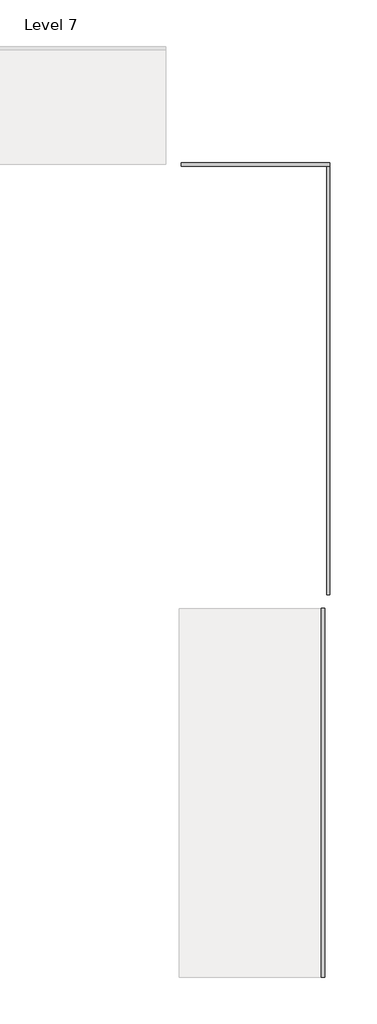
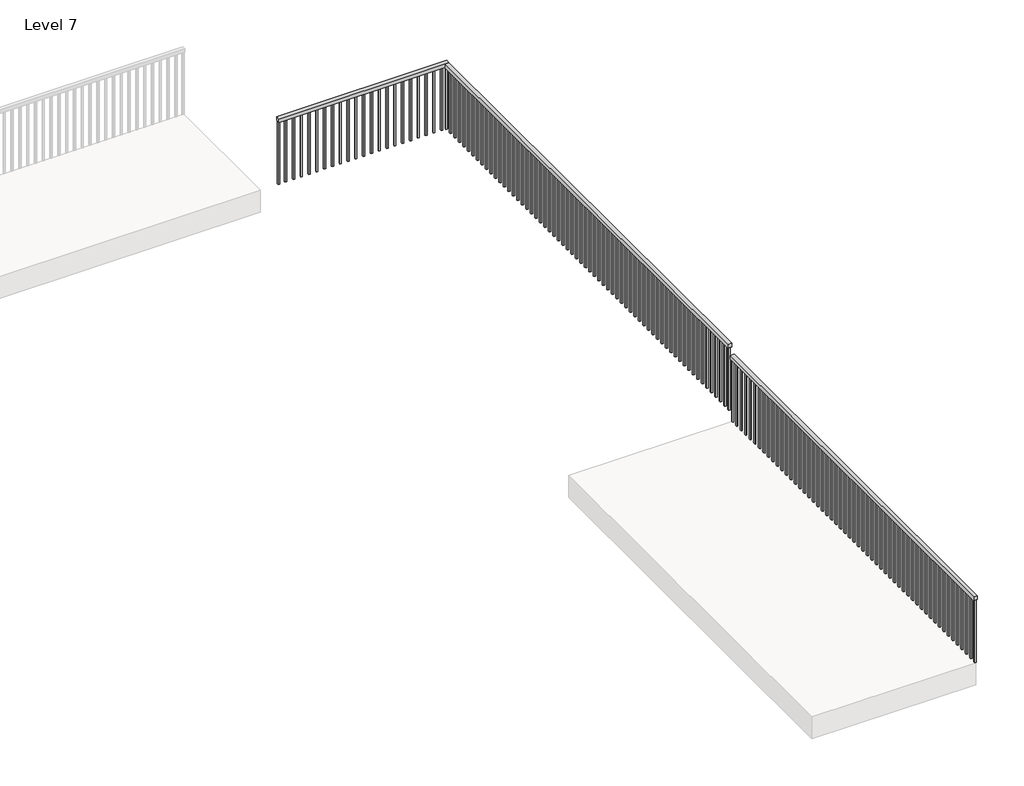
# One storey, part 4 of 5: 3 railings.
"""IFC4 building model written with IfcOpenShell, lengths in millimetres."""

from ifc_helpers import new_model, si_unit, frame, origin, place, context, project, spatial, polyline, outline, extrude, element, save

model = new_model("IFC4")

# Units and contexts
model_context = context("Model", 3, world=origin())
ifc_project = project(units=[si_unit("LENGTHUNIT", "METRE", prefix="MILLI")], contexts=[model_context])

# Site, building, storey
site = spatial("IfcSite", under=ifc_project)
building = spatial("IfcBuilding", under=site)
storey = spatial("IfcBuildingStorey", under=building, Name="Level 7", Elevation=6400.8)

# Railings
placement = place(None, origin())
element("IfcRailing", 1, ObjectType="Handrail - Rectangular", at=placement, inside=storey, context=model_context, shape_type="SweptSolid", body=[
    extrude(outline(polyline([(16346.8289933, 8367.8237525), (16296.0289933, 8367.8237525), (16296.0289933, 14768.6237525), (16346.8289933, 14768.6237525), (16346.8289933, 8367.8237525)])), frame((0.0, 0.0, 7264.4), z_axis=(0.0, 0.0, 1.0), x_axis=(1.0, 0.0, 0.0)), (0.0, 0.0, 1.0), 50.8),
    extrude(outline(polyline([(16330.9539933, 14657.4987525), (16311.9039933, 14657.4987525), (16311.9039933, 14676.5487525), (16330.9539933, 14676.5487525), (16330.9539933, 14657.4987525)])), frame((0.0, 0.0, 6400.8), z_axis=(0.0, 0.0, 1.0), x_axis=(1.0, 0.0, 0.0)), (0.0, 0.0, 1.0), 863.6),
    extrude(outline(polyline([(16330.9539933, 14555.8987525), (16311.9039933, 14555.8987525), (16311.9039933, 14574.9487525), (16330.9539933, 14574.9487525), (16330.9539933, 14555.8987525)])), frame((0.0, 0.0, 6400.8), z_axis=(0.0, 0.0, 1.0), x_axis=(1.0, 0.0, 0.0)), (0.0, 0.0, 1.0), 863.6),
    extrude(outline(polyline([(16330.9539933, 14454.2987525), (16311.9039933, 14454.2987525), (16311.9039933, 14473.3487525), (16330.9539933, 14473.3487525), (16330.9539933, 14454.2987525)])), frame((0.0, 0.0, 6400.8), z_axis=(0.0, 0.0, 1.0), x_axis=(1.0, 0.0, 0.0)), (0.0, 0.0, 1.0), 863.6),
    extrude(outline(polyline([(16330.9539933, 14352.6987525), (16311.9039933, 14352.6987525), (16311.9039933, 14371.7487525), (16330.9539933, 14371.7487525), (16330.9539933, 14352.6987525)])), frame((0.0, 0.0, 6400.8), z_axis=(0.0, 0.0, 1.0), x_axis=(1.0, 0.0, 0.0)), (0.0, 0.0, 1.0), 863.6),
    extrude(outline(polyline([(16330.9539933, 14251.0987525), (16311.9039933, 14251.0987525), (16311.9039933, 14270.1487525), (16330.9539933, 14270.1487525), (16330.9539933, 14251.0987525)])), frame((0.0, 0.0, 6400.8), z_axis=(0.0, 0.0, 1.0), x_axis=(1.0, 0.0, 0.0)), (0.0, 0.0, 1.0), 863.6),
    extrude(outline(polyline([(16330.9539933, 14149.4987525), (16311.9039933, 14149.4987525), (16311.9039933, 14168.5487525), (16330.9539933, 14168.5487525), (16330.9539933, 14149.4987525)])), frame((0.0, 0.0, 6400.8), z_axis=(0.0, 0.0, 1.0), x_axis=(1.0, 0.0, 0.0)), (0.0, 0.0, 1.0), 863.6),
    extrude(outline(polyline([(16330.9539933, 14047.8987525), (16311.9039933, 14047.8987525), (16311.9039933, 14066.9487525), (16330.9539933, 14066.9487525), (16330.9539933, 14047.8987525)])), frame((0.0, 0.0, 6400.8), z_axis=(0.0, 0.0, 1.0), x_axis=(1.0, 0.0, 0.0)), (0.0, 0.0, 1.0), 863.6),
    extrude(outline(polyline([(16330.9539933, 13946.2987525), (16311.9039933, 13946.2987525), (16311.9039933, 13965.3487525), (16330.9539933, 13965.3487525), (16330.9539933, 13946.2987525)])), frame((0.0, 0.0, 6400.8), z_axis=(0.0, 0.0, 1.0), x_axis=(1.0, 0.0, 0.0)), (0.0, 0.0, 1.0), 863.6),
    extrude(outline(polyline([(16330.9539933, 13844.6987525), (16311.9039933, 13844.6987525), (16311.9039933, 13863.7487525), (16330.9539933, 13863.7487525), (16330.9539933, 13844.6987525)])), frame((0.0, 0.0, 6400.8), z_axis=(0.0, 0.0, 1.0), x_axis=(1.0, 0.0, 0.0)), (0.0, 0.0, 1.0), 863.6),
    extrude(outline(polyline([(16330.9539933, 13743.0987525), (16311.9039933, 13743.0987525), (16311.9039933, 13762.1487525), (16330.9539933, 13762.1487525), (16330.9539933, 13743.0987525)])), frame((0.0, 0.0, 6400.8), z_axis=(0.0, 0.0, 1.0), x_axis=(1.0, 0.0, 0.0)), (0.0, 0.0, 1.0), 863.6),
    extrude(outline(polyline([(16330.9539933, 13641.4987525), (16311.9039933, 13641.4987525), (16311.9039933, 13660.5487525), (16330.9539933, 13660.5487525), (16330.9539933, 13641.4987525)])), frame((0.0, 0.0, 6400.8), z_axis=(0.0, 0.0, 1.0), x_axis=(1.0, 0.0, 0.0)), (0.0, 0.0, 1.0), 863.6),
    extrude(outline(polyline([(16330.9539933, 13539.8987525), (16311.9039933, 13539.8987525), (16311.9039933, 13558.9487525), (16330.9539933, 13558.9487525), (16330.9539933, 13539.8987525)])), frame((0.0, 0.0, 6400.8), z_axis=(0.0, 0.0, 1.0), x_axis=(1.0, 0.0, 0.0)), (0.0, 0.0, 1.0), 863.6),
    extrude(outline(polyline([(16330.9539933, 13438.2987525), (16311.9039933, 13438.2987525), (16311.9039933, 13457.3487525), (16330.9539933, 13457.3487525), (16330.9539933, 13438.2987525)])), frame((0.0, 0.0, 6400.8), z_axis=(0.0, 0.0, 1.0), x_axis=(1.0, 0.0, 0.0)), (0.0, 0.0, 1.0), 863.6),
    extrude(outline(polyline([(16330.9539933, 13336.6987525), (16311.9039933, 13336.6987525), (16311.9039933, 13355.7487525), (16330.9539933, 13355.7487525), (16330.9539933, 13336.6987525)])), frame((0.0, 0.0, 6400.8), z_axis=(0.0, 0.0, 1.0), x_axis=(1.0, 0.0, 0.0)), (0.0, 0.0, 1.0), 863.6),
    extrude(outline(polyline([(16330.9539933, 13235.0987525), (16311.9039933, 13235.0987525), (16311.9039933, 13254.1487525), (16330.9539933, 13254.1487525), (16330.9539933, 13235.0987525)])), frame((0.0, 0.0, 6400.8), z_axis=(0.0, 0.0, 1.0), x_axis=(1.0, 0.0, 0.0)), (0.0, 0.0, 1.0), 863.6),
    extrude(outline(polyline([(16330.9539933, 13133.4987525), (16311.9039933, 13133.4987525), (16311.9039933, 13152.5487525), (16330.9539933, 13152.5487525), (16330.9539933, 13133.4987525)])), frame((0.0, 0.0, 6400.8), z_axis=(0.0, 0.0, 1.0), x_axis=(1.0, 0.0, 0.0)), (0.0, 0.0, 1.0), 863.6),
    extrude(outline(polyline([(16330.9539933, 13031.8987525), (16311.9039933, 13031.8987525), (16311.9039933, 13050.9487525), (16330.9539933, 13050.9487525), (16330.9539933, 13031.8987525)])), frame((0.0, 0.0, 6400.8), z_axis=(0.0, 0.0, 1.0), x_axis=(1.0, 0.0, 0.0)), (0.0, 0.0, 1.0), 863.6),
    extrude(outline(polyline([(16330.9539933, 12930.2987525), (16311.9039933, 12930.2987525), (16311.9039933, 12949.3487525), (16330.9539933, 12949.3487525), (16330.9539933, 12930.2987525)])), frame((0.0, 0.0, 6400.8), z_axis=(0.0, 0.0, 1.0), x_axis=(1.0, 0.0, 0.0)), (0.0, 0.0, 1.0), 863.6),
    extrude(outline(polyline([(16330.9539933, 12828.6987525), (16311.9039933, 12828.6987525), (16311.9039933, 12847.7487525), (16330.9539933, 12847.7487525), (16330.9539933, 12828.6987525)])), frame((0.0, 0.0, 6400.8), z_axis=(0.0, 0.0, 1.0), x_axis=(1.0, 0.0, 0.0)), (0.0, 0.0, 1.0), 863.6),
    extrude(outline(polyline([(16330.9539933, 12727.0987525), (16311.9039933, 12727.0987525), (16311.9039933, 12746.1487525), (16330.9539933, 12746.1487525), (16330.9539933, 12727.0987525)])), frame((0.0, 0.0, 6400.8), z_axis=(0.0, 0.0, 1.0), x_axis=(1.0, 0.0, 0.0)), (0.0, 0.0, 1.0), 863.6),
    extrude(outline(polyline([(16330.9539933, 12625.4987525), (16311.9039933, 12625.4987525), (16311.9039933, 12644.5487525), (16330.9539933, 12644.5487525), (16330.9539933, 12625.4987525)])), frame((0.0, 0.0, 6400.8), z_axis=(0.0, 0.0, 1.0), x_axis=(1.0, 0.0, 0.0)), (0.0, 0.0, 1.0), 863.6),
    extrude(outline(polyline([(16330.9539933, 12523.8987525), (16311.9039933, 12523.8987525), (16311.9039933, 12542.9487525), (16330.9539933, 12542.9487525), (16330.9539933, 12523.8987525)])), frame((0.0, 0.0, 6400.8), z_axis=(0.0, 0.0, 1.0), x_axis=(1.0, 0.0, 0.0)), (0.0, 0.0, 1.0), 863.6),
    extrude(outline(polyline([(16330.9539933, 12422.2987525), (16311.9039933, 12422.2987525), (16311.9039933, 12441.3487525), (16330.9539933, 12441.3487525), (16330.9539933, 12422.2987525)])), frame((0.0, 0.0, 6400.8), z_axis=(0.0, 0.0, 1.0), x_axis=(1.0, 0.0, 0.0)), (0.0, 0.0, 1.0), 863.6),
    extrude(outline(polyline([(16330.9539933, 12320.6987525), (16311.9039933, 12320.6987525), (16311.9039933, 12339.7487525), (16330.9539933, 12339.7487525), (16330.9539933, 12320.6987525)])), frame((0.0, 0.0, 6400.8), z_axis=(0.0, 0.0, 1.0), x_axis=(1.0, 0.0, 0.0)), (0.0, 0.0, 1.0), 863.6),
    extrude(outline(polyline([(16330.9539933, 12219.0987525), (16311.9039933, 12219.0987525), (16311.9039933, 12238.1487525), (16330.9539933, 12238.1487525), (16330.9539933, 12219.0987525)])), frame((0.0, 0.0, 6400.8), z_axis=(0.0, 0.0, 1.0), x_axis=(1.0, 0.0, 0.0)), (0.0, 0.0, 1.0), 863.6),
    extrude(outline(polyline([(16330.9539933, 12117.4987525), (16311.9039933, 12117.4987525), (16311.9039933, 12136.5487525), (16330.9539933, 12136.5487525), (16330.9539933, 12117.4987525)])), frame((0.0, 0.0, 6400.8), z_axis=(0.0, 0.0, 1.0), x_axis=(1.0, 0.0, 0.0)), (0.0, 0.0, 1.0), 863.6),
    extrude(outline(polyline([(16330.9539933, 12015.8987525), (16311.9039933, 12015.8987525), (16311.9039933, 12034.9487525), (16330.9539933, 12034.9487525), (16330.9539933, 12015.8987525)])), frame((0.0, 0.0, 6400.8), z_axis=(0.0, 0.0, 1.0), x_axis=(1.0, 0.0, 0.0)), (0.0, 0.0, 1.0), 863.6),
    extrude(outline(polyline([(16330.9539933, 11914.2987525), (16311.9039933, 11914.2987525), (16311.9039933, 11933.3487525), (16330.9539933, 11933.3487525), (16330.9539933, 11914.2987525)])), frame((0.0, 0.0, 6400.8), z_axis=(0.0, 0.0, 1.0), x_axis=(1.0, 0.0, 0.0)), (0.0, 0.0, 1.0), 863.6),
    extrude(outline(polyline([(16330.9539933, 11812.6987525), (16311.9039933, 11812.6987525), (16311.9039933, 11831.7487525), (16330.9539933, 11831.7487525), (16330.9539933, 11812.6987525)])), frame((0.0, 0.0, 6400.8), z_axis=(0.0, 0.0, 1.0), x_axis=(1.0, 0.0, 0.0)), (0.0, 0.0, 1.0), 863.6),
    extrude(outline(polyline([(16330.9539933, 11711.0987525), (16311.9039933, 11711.0987525), (16311.9039933, 11730.1487525), (16330.9539933, 11730.1487525), (16330.9539933, 11711.0987525)])), frame((0.0, 0.0, 6400.8), z_axis=(0.0, 0.0, 1.0), x_axis=(1.0, 0.0, 0.0)), (0.0, 0.0, 1.0), 863.6),
    extrude(outline(polyline([(16330.9539933, 11609.4987525), (16311.9039933, 11609.4987525), (16311.9039933, 11628.5487525), (16330.9539933, 11628.5487525), (16330.9539933, 11609.4987525)])), frame((0.0, 0.0, 6400.8), z_axis=(0.0, 0.0, 1.0), x_axis=(1.0, 0.0, 0.0)), (0.0, 0.0, 1.0), 863.6),
    extrude(outline(polyline([(16330.9539933, 11507.8987525), (16311.9039933, 11507.8987525), (16311.9039933, 11526.9487525), (16330.9539933, 11526.9487525), (16330.9539933, 11507.8987525)])), frame((0.0, 0.0, 6400.8), z_axis=(0.0, 0.0, 1.0), x_axis=(1.0, 0.0, 0.0)), (0.0, 0.0, 1.0), 863.6),
    extrude(outline(polyline([(16330.9539933, 11406.2987525), (16311.9039933, 11406.2987525), (16311.9039933, 11425.3487525), (16330.9539933, 11425.3487525), (16330.9539933, 11406.2987525)])), frame((0.0, 0.0, 6400.8), z_axis=(0.0, 0.0, 1.0), x_axis=(1.0, 0.0, 0.0)), (0.0, 0.0, 1.0), 863.6),
    extrude(outline(polyline([(16330.9539933, 11304.6987525), (16311.9039933, 11304.6987525), (16311.9039933, 11323.7487525), (16330.9539933, 11323.7487525), (16330.9539933, 11304.6987525)])), frame((0.0, 0.0, 6400.8), z_axis=(0.0, 0.0, 1.0), x_axis=(1.0, 0.0, 0.0)), (0.0, 0.0, 1.0), 863.6),
    extrude(outline(polyline([(16330.9539933, 11203.0987525), (16311.9039933, 11203.0987525), (16311.9039933, 11222.1487525), (16330.9539933, 11222.1487525), (16330.9539933, 11203.0987525)])), frame((0.0, 0.0, 6400.8), z_axis=(0.0, 0.0, 1.0), x_axis=(1.0, 0.0, 0.0)), (0.0, 0.0, 1.0), 863.6),
    extrude(outline(polyline([(16330.9539933, 11101.4987525), (16311.9039933, 11101.4987525), (16311.9039933, 11120.5487525), (16330.9539933, 11120.5487525), (16330.9539933, 11101.4987525)])), frame((0.0, 0.0, 6400.8), z_axis=(0.0, 0.0, 1.0), x_axis=(1.0, 0.0, 0.0)), (0.0, 0.0, 1.0), 863.6),
    extrude(outline(polyline([(16330.9539933, 10999.8987525), (16311.9039933, 10999.8987525), (16311.9039933, 11018.9487525), (16330.9539933, 11018.9487525), (16330.9539933, 10999.8987525)])), frame((0.0, 0.0, 6400.8), z_axis=(0.0, 0.0, 1.0), x_axis=(1.0, 0.0, 0.0)), (0.0, 0.0, 1.0), 863.6),
    extrude(outline(polyline([(16330.9539933, 10898.2987525), (16311.9039933, 10898.2987525), (16311.9039933, 10917.3487525), (16330.9539933, 10917.3487525), (16330.9539933, 10898.2987525)])), frame((0.0, 0.0, 6400.8), z_axis=(0.0, 0.0, 1.0), x_axis=(1.0, 0.0, 0.0)), (0.0, 0.0, 1.0), 863.6),
    extrude(outline(polyline([(16330.9539933, 10796.6987525), (16311.9039933, 10796.6987525), (16311.9039933, 10815.7487525), (16330.9539933, 10815.7487525), (16330.9539933, 10796.6987525)])), frame((0.0, 0.0, 6400.8), z_axis=(0.0, 0.0, 1.0), x_axis=(1.0, 0.0, 0.0)), (0.0, 0.0, 1.0), 863.6),
    extrude(outline(polyline([(16330.9539933, 10695.0987525), (16311.9039933, 10695.0987525), (16311.9039933, 10714.1487525), (16330.9539933, 10714.1487525), (16330.9539933, 10695.0987525)])), frame((0.0, 0.0, 6400.8), z_axis=(0.0, 0.0, 1.0), x_axis=(1.0, 0.0, 0.0)), (0.0, 0.0, 1.0), 863.6),
    extrude(outline(polyline([(16330.9539933, 10593.4987525), (16311.9039933, 10593.4987525), (16311.9039933, 10612.5487525), (16330.9539933, 10612.5487525), (16330.9539933, 10593.4987525)])), frame((0.0, 0.0, 6400.8), z_axis=(0.0, 0.0, 1.0), x_axis=(1.0, 0.0, 0.0)), (0.0, 0.0, 1.0), 863.6),
    extrude(outline(polyline([(16330.9539933, 10491.8987525), (16311.9039933, 10491.8987525), (16311.9039933, 10510.9487525), (16330.9539933, 10510.9487525), (16330.9539933, 10491.8987525)])), frame((0.0, 0.0, 6400.8), z_axis=(0.0, 0.0, 1.0), x_axis=(1.0, 0.0, 0.0)), (0.0, 0.0, 1.0), 863.6),
    extrude(outline(polyline([(16330.9539933, 10390.2987525), (16311.9039933, 10390.2987525), (16311.9039933, 10409.3487525), (16330.9539933, 10409.3487525), (16330.9539933, 10390.2987525)])), frame((0.0, 0.0, 6400.8), z_axis=(0.0, 0.0, 1.0), x_axis=(1.0, 0.0, 0.0)), (0.0, 0.0, 1.0), 863.6),
    extrude(outline(polyline([(16330.9539933, 10288.6987525), (16311.9039933, 10288.6987525), (16311.9039933, 10307.7487525), (16330.9539933, 10307.7487525), (16330.9539933, 10288.6987525)])), frame((0.0, 0.0, 6400.8), z_axis=(0.0, 0.0, 1.0), x_axis=(1.0, 0.0, 0.0)), (0.0, 0.0, 1.0), 863.6),
    extrude(outline(polyline([(16330.9539933, 10187.0987525), (16311.9039933, 10187.0987525), (16311.9039933, 10206.1487525), (16330.9539933, 10206.1487525), (16330.9539933, 10187.0987525)])), frame((0.0, 0.0, 6400.8), z_axis=(0.0, 0.0, 1.0), x_axis=(1.0, 0.0, 0.0)), (0.0, 0.0, 1.0), 863.6),
    extrude(outline(polyline([(16330.9539933, 10085.4987525), (16311.9039933, 10085.4987525), (16311.9039933, 10104.5487525), (16330.9539933, 10104.5487525), (16330.9539933, 10085.4987525)])), frame((0.0, 0.0, 6400.8), z_axis=(0.0, 0.0, 1.0), x_axis=(1.0, 0.0, 0.0)), (0.0, 0.0, 1.0), 863.6),
    extrude(outline(polyline([(16330.9539933, 9983.8987525), (16311.9039933, 9983.8987525), (16311.9039933, 10002.9487525), (16330.9539933, 10002.9487525), (16330.9539933, 9983.8987525)])), frame((0.0, 0.0, 6400.8), z_axis=(0.0, 0.0, 1.0), x_axis=(1.0, 0.0, 0.0)), (0.0, 0.0, 1.0), 863.6),
    extrude(outline(polyline([(16330.9539933, 9882.2987525), (16311.9039933, 9882.2987525), (16311.9039933, 9901.3487525), (16330.9539933, 9901.3487525), (16330.9539933, 9882.2987525)])), frame((0.0, 0.0, 6400.8), z_axis=(0.0, 0.0, 1.0), x_axis=(1.0, 0.0, 0.0)), (0.0, 0.0, 1.0), 863.6),
    extrude(outline(polyline([(16330.9539933, 9780.6987525), (16311.9039933, 9780.6987525), (16311.9039933, 9799.7487525), (16330.9539933, 9799.7487525), (16330.9539933, 9780.6987525)])), frame((0.0, 0.0, 6400.8), z_axis=(0.0, 0.0, 1.0), x_axis=(1.0, 0.0, 0.0)), (0.0, 0.0, 1.0), 863.6),
    extrude(outline(polyline([(16330.9539933, 9679.0987525), (16311.9039933, 9679.0987525), (16311.9039933, 9698.1487525), (16330.9539933, 9698.1487525), (16330.9539933, 9679.0987525)])), frame((0.0, 0.0, 6400.8), z_axis=(0.0, 0.0, 1.0), x_axis=(1.0, 0.0, 0.0)), (0.0, 0.0, 1.0), 863.6),
    extrude(outline(polyline([(16330.9539933, 9577.4987525), (16311.9039933, 9577.4987525), (16311.9039933, 9596.5487525), (16330.9539933, 9596.5487525), (16330.9539933, 9577.4987525)])), frame((0.0, 0.0, 6400.8), z_axis=(0.0, 0.0, 1.0), x_axis=(1.0, 0.0, 0.0)), (0.0, 0.0, 1.0), 863.6),
    extrude(outline(polyline([(16330.9539933, 9475.8987525), (16311.9039933, 9475.8987525), (16311.9039933, 9494.9487525), (16330.9539933, 9494.9487525), (16330.9539933, 9475.8987525)])), frame((0.0, 0.0, 6400.8), z_axis=(0.0, 0.0, 1.0), x_axis=(1.0, 0.0, 0.0)), (0.0, 0.0, 1.0), 863.6),
    extrude(outline(polyline([(16330.9539933, 9374.2987525), (16311.9039933, 9374.2987525), (16311.9039933, 9393.3487525), (16330.9539933, 9393.3487525), (16330.9539933, 9374.2987525)])), frame((0.0, 0.0, 6400.8), z_axis=(0.0, 0.0, 1.0), x_axis=(1.0, 0.0, 0.0)), (0.0, 0.0, 1.0), 863.6),
    extrude(outline(polyline([(16330.9539933, 9272.6987525), (16311.9039933, 9272.6987525), (16311.9039933, 9291.7487525), (16330.9539933, 9291.7487525), (16330.9539933, 9272.6987525)])), frame((0.0, 0.0, 6400.8), z_axis=(0.0, 0.0, 1.0), x_axis=(1.0, 0.0, 0.0)), (0.0, 0.0, 1.0), 863.6),
    extrude(outline(polyline([(16330.9539933, 9171.0987525), (16311.9039933, 9171.0987525), (16311.9039933, 9190.1487525), (16330.9539933, 9190.1487525), (16330.9539933, 9171.0987525)])), frame((0.0, 0.0, 6400.8), z_axis=(0.0, 0.0, 1.0), x_axis=(1.0, 0.0, 0.0)), (0.0, 0.0, 1.0), 863.6),
    extrude(outline(polyline([(16330.9539933, 9069.4987525), (16311.9039933, 9069.4987525), (16311.9039933, 9088.5487525), (16330.9539933, 9088.5487525), (16330.9539933, 9069.4987525)])), frame((0.0, 0.0, 6400.8), z_axis=(0.0, 0.0, 1.0), x_axis=(1.0, 0.0, 0.0)), (0.0, 0.0, 1.0), 863.6),
    extrude(outline(polyline([(16330.9539933, 8967.8987525), (16311.9039933, 8967.8987525), (16311.9039933, 8986.9487525), (16330.9539933, 8986.9487525), (16330.9539933, 8967.8987525)])), frame((0.0, 0.0, 6400.8), z_axis=(0.0, 0.0, 1.0), x_axis=(1.0, 0.0, 0.0)), (0.0, 0.0, 1.0), 863.6),
    extrude(outline(polyline([(16330.9539933, 8866.2987525), (16311.9039933, 8866.2987525), (16311.9039933, 8885.3487525), (16330.9539933, 8885.3487525), (16330.9539933, 8866.2987525)])), frame((0.0, 0.0, 6400.8), z_axis=(0.0, 0.0, 1.0), x_axis=(1.0, 0.0, 0.0)), (0.0, 0.0, 1.0), 863.6),
    extrude(outline(polyline([(16330.9539933, 8764.6987525), (16311.9039933, 8764.6987525), (16311.9039933, 8783.7487525), (16330.9539933, 8783.7487525), (16330.9539933, 8764.6987525)])), frame((0.0, 0.0, 6400.8), z_axis=(0.0, 0.0, 1.0), x_axis=(1.0, 0.0, 0.0)), (0.0, 0.0, 1.0), 863.6),
    extrude(outline(polyline([(16330.9539933, 8663.0987525), (16311.9039933, 8663.0987525), (16311.9039933, 8682.1487525), (16330.9539933, 8682.1487525), (16330.9539933, 8663.0987525)])), frame((0.0, 0.0, 6400.8), z_axis=(0.0, 0.0, 1.0), x_axis=(1.0, 0.0, 0.0)), (0.0, 0.0, 1.0), 863.6),
    extrude(outline(polyline([(16330.9539933, 8561.4987525), (16311.9039933, 8561.4987525), (16311.9039933, 8580.5487525), (16330.9539933, 8580.5487525), (16330.9539933, 8561.4987525)])), frame((0.0, 0.0, 6400.8), z_axis=(0.0, 0.0, 1.0), x_axis=(1.0, 0.0, 0.0)), (0.0, 0.0, 1.0), 863.6),
    extrude(outline(polyline([(16330.9539933, 8459.8987525), (16311.9039933, 8459.8987525), (16311.9039933, 8478.9487525), (16330.9539933, 8478.9487525), (16330.9539933, 8459.8987525)])), frame((0.0, 0.0, 6400.8), z_axis=(0.0, 0.0, 1.0), x_axis=(1.0, 0.0, 0.0)), (0.0, 0.0, 1.0), 863.6),
    extrude(outline(polyline([(16330.9539933, 14749.5737525), (16311.9039933, 14749.5737525), (16311.9039933, 14768.6237525), (16330.9539933, 14768.6237525), (16330.9539933, 14749.5737525)])), frame((0.0, 0.0, 6400.8), z_axis=(0.0, 0.0, 1.0), x_axis=(1.0, 0.0, 0.0)), (0.0, 0.0, 1.0), 863.6),
    extrude(outline(polyline([(16330.9539933, 8367.8237525), (16311.9039933, 8367.8237525), (16311.9039933, 8386.8737525), (16330.9539933, 8386.8737525), (16330.9539933, 8367.8237525)])), frame((0.0, 0.0, 6400.8), z_axis=(0.0, 0.0, 1.0), x_axis=(1.0, 0.0, 0.0)), (0.0, 0.0, 1.0), 863.6),
])
element("IfcRailing", 2, ObjectType="Handrail - Rectangular", at=placement, inside=storey, context=model_context, shape_type="SweptSolid", body=[
    extrude(outline(polyline([(14131.9361222, 14743.2237525), (14131.9361222, 14794.0237525), (16346.8289933, 14794.0237525), (16346.8289933, 14743.2237525), (14131.9361222, 14743.2237525)])), frame((0.0, 0.0, 7264.4), z_axis=(0.0, 0.0, 1.0), x_axis=(1.0, 0.0, 0.0)), (0.0, 0.0, 1.0), 50.8),
    extrude(outline(polyline([(16256.0111222, 14759.0987525), (16256.0111222, 14778.1487525), (16275.0611222, 14778.1487525), (16275.0611222, 14759.0987525), (16256.0111222, 14759.0987525)])), frame((0.0, 0.0, 6400.8), z_axis=(0.0, 0.0, 1.0), x_axis=(1.0, 0.0, 0.0)), (0.0, 0.0, 1.0), 863.6),
    extrude(outline(polyline([(16154.4111222, 14759.0987525), (16154.4111222, 14778.1487525), (16173.4611222, 14778.1487525), (16173.4611222, 14759.0987525), (16154.4111222, 14759.0987525)])), frame((0.0, 0.0, 6400.8), z_axis=(0.0, 0.0, 1.0), x_axis=(1.0, 0.0, 0.0)), (0.0, 0.0, 1.0), 863.6),
    extrude(outline(polyline([(16052.8111222, 14759.0987525), (16052.8111222, 14778.1487525), (16071.8611222, 14778.1487525), (16071.8611222, 14759.0987525), (16052.8111222, 14759.0987525)])), frame((0.0, 0.0, 6400.8), z_axis=(0.0, 0.0, 1.0), x_axis=(1.0, 0.0, 0.0)), (0.0, 0.0, 1.0), 863.6),
    extrude(outline(polyline([(15951.2111222, 14759.0987525), (15951.2111222, 14778.1487525), (15970.2611222, 14778.1487525), (15970.2611222, 14759.0987525), (15951.2111222, 14759.0987525)])), frame((0.0, 0.0, 6400.8), z_axis=(0.0, 0.0, 1.0), x_axis=(1.0, 0.0, 0.0)), (0.0, 0.0, 1.0), 863.6),
    extrude(outline(polyline([(15849.6111222, 14759.0987525), (15849.6111222, 14778.1487525), (15868.6611222, 14778.1487525), (15868.6611222, 14759.0987525), (15849.6111222, 14759.0987525)])), frame((0.0, 0.0, 6400.8), z_axis=(0.0, 0.0, 1.0), x_axis=(1.0, 0.0, 0.0)), (0.0, 0.0, 1.0), 863.6),
    extrude(outline(polyline([(15748.0111222, 14759.0987525), (15748.0111222, 14778.1487525), (15767.0611222, 14778.1487525), (15767.0611222, 14759.0987525), (15748.0111222, 14759.0987525)])), frame((0.0, 0.0, 6400.8), z_axis=(0.0, 0.0, 1.0), x_axis=(1.0, 0.0, 0.0)), (0.0, 0.0, 1.0), 863.6),
    extrude(outline(polyline([(15646.4111222, 14759.0987525), (15646.4111222, 14778.1487525), (15665.4611222, 14778.1487525), (15665.4611222, 14759.0987525), (15646.4111222, 14759.0987525)])), frame((0.0, 0.0, 6400.8), z_axis=(0.0, 0.0, 1.0), x_axis=(1.0, 0.0, 0.0)), (0.0, 0.0, 1.0), 863.6),
    extrude(outline(polyline([(15544.8111222, 14759.0987525), (15544.8111222, 14778.1487525), (15563.8611222, 14778.1487525), (15563.8611222, 14759.0987525), (15544.8111222, 14759.0987525)])), frame((0.0, 0.0, 6400.8), z_axis=(0.0, 0.0, 1.0), x_axis=(1.0, 0.0, 0.0)), (0.0, 0.0, 1.0), 863.6),
    extrude(outline(polyline([(15443.2111222, 14759.0987525), (15443.2111222, 14778.1487525), (15462.2611222, 14778.1487525), (15462.2611222, 14759.0987525), (15443.2111222, 14759.0987525)])), frame((0.0, 0.0, 6400.8), z_axis=(0.0, 0.0, 1.0), x_axis=(1.0, 0.0, 0.0)), (0.0, 0.0, 1.0), 863.6),
    extrude(outline(polyline([(15341.6111222, 14759.0987525), (15341.6111222, 14778.1487525), (15360.6611222, 14778.1487525), (15360.6611222, 14759.0987525), (15341.6111222, 14759.0987525)])), frame((0.0, 0.0, 6400.8), z_axis=(0.0, 0.0, 1.0), x_axis=(1.0, 0.0, 0.0)), (0.0, 0.0, 1.0), 863.6),
    extrude(outline(polyline([(15240.0111222, 14759.0987525), (15240.0111222, 14778.1487525), (15259.0611222, 14778.1487525), (15259.0611222, 14759.0987525), (15240.0111222, 14759.0987525)])), frame((0.0, 0.0, 6400.8), z_axis=(0.0, 0.0, 1.0), x_axis=(1.0, 0.0, 0.0)), (0.0, 0.0, 1.0), 863.6),
    extrude(outline(polyline([(15138.4111222, 14759.0987525), (15138.4111222, 14778.1487525), (15157.4611222, 14778.1487525), (15157.4611222, 14759.0987525), (15138.4111222, 14759.0987525)])), frame((0.0, 0.0, 6400.8), z_axis=(0.0, 0.0, 1.0), x_axis=(1.0, 0.0, 0.0)), (0.0, 0.0, 1.0), 863.6),
    extrude(outline(polyline([(15036.8111222, 14759.0987525), (15036.8111222, 14778.1487525), (15055.8611222, 14778.1487525), (15055.8611222, 14759.0987525), (15036.8111222, 14759.0987525)])), frame((0.0, 0.0, 6400.8), z_axis=(0.0, 0.0, 1.0), x_axis=(1.0, 0.0, 0.0)), (0.0, 0.0, 1.0), 863.6),
    extrude(outline(polyline([(14935.2111222, 14759.0987525), (14935.2111222, 14778.1487525), (14954.2611222, 14778.1487525), (14954.2611222, 14759.0987525), (14935.2111222, 14759.0987525)])), frame((0.0, 0.0, 6400.8), z_axis=(0.0, 0.0, 1.0), x_axis=(1.0, 0.0, 0.0)), (0.0, 0.0, 1.0), 863.6),
    extrude(outline(polyline([(14833.6111222, 14759.0987525), (14833.6111222, 14778.1487525), (14852.6611222, 14778.1487525), (14852.6611222, 14759.0987525), (14833.6111222, 14759.0987525)])), frame((0.0, 0.0, 6400.8), z_axis=(0.0, 0.0, 1.0), x_axis=(1.0, 0.0, 0.0)), (0.0, 0.0, 1.0), 863.6),
    extrude(outline(polyline([(14732.0111222, 14759.0987525), (14732.0111222, 14778.1487525), (14751.0611222, 14778.1487525), (14751.0611222, 14759.0987525), (14732.0111222, 14759.0987525)])), frame((0.0, 0.0, 6400.8), z_axis=(0.0, 0.0, 1.0), x_axis=(1.0, 0.0, 0.0)), (0.0, 0.0, 1.0), 863.6),
    extrude(outline(polyline([(14630.4111222, 14759.0987525), (14630.4111222, 14778.1487525), (14649.4611222, 14778.1487525), (14649.4611222, 14759.0987525), (14630.4111222, 14759.0987525)])), frame((0.0, 0.0, 6400.8), z_axis=(0.0, 0.0, 1.0), x_axis=(1.0, 0.0, 0.0)), (0.0, 0.0, 1.0), 863.6),
    extrude(outline(polyline([(14528.8111222, 14759.0987525), (14528.8111222, 14778.1487525), (14547.8611222, 14778.1487525), (14547.8611222, 14759.0987525), (14528.8111222, 14759.0987525)])), frame((0.0, 0.0, 6400.8), z_axis=(0.0, 0.0, 1.0), x_axis=(1.0, 0.0, 0.0)), (0.0, 0.0, 1.0), 863.6),
    extrude(outline(polyline([(14427.2111222, 14759.0987525), (14427.2111222, 14778.1487525), (14446.2611222, 14778.1487525), (14446.2611222, 14759.0987525), (14427.2111222, 14759.0987525)])), frame((0.0, 0.0, 6400.8), z_axis=(0.0, 0.0, 1.0), x_axis=(1.0, 0.0, 0.0)), (0.0, 0.0, 1.0), 863.6),
    extrude(outline(polyline([(14325.6111222, 14759.0987525), (14325.6111222, 14778.1487525), (14344.6611222, 14778.1487525), (14344.6611222, 14759.0987525), (14325.6111222, 14759.0987525)])), frame((0.0, 0.0, 6400.8), z_axis=(0.0, 0.0, 1.0), x_axis=(1.0, 0.0, 0.0)), (0.0, 0.0, 1.0), 863.6),
    extrude(outline(polyline([(14224.0111222, 14759.0987525), (14224.0111222, 14778.1487525), (14243.0611222, 14778.1487525), (14243.0611222, 14759.0987525), (14224.0111222, 14759.0987525)])), frame((0.0, 0.0, 6400.8), z_axis=(0.0, 0.0, 1.0), x_axis=(1.0, 0.0, 0.0)), (0.0, 0.0, 1.0), 863.6),
    extrude(outline(polyline([(16327.7789933, 14759.0987525), (16327.7789933, 14778.1487525), (16346.8289933, 14778.1487525), (16346.8289933, 14759.0987525), (16327.7789933, 14759.0987525)])), frame((0.0, 0.0, 6400.8), z_axis=(0.0, 0.0, 1.0), x_axis=(1.0, 0.0, 0.0)), (0.0, 0.0, 1.0), 863.6),
    extrude(outline(polyline([(14131.9361222, 14759.0987525), (14131.9361222, 14778.1487525), (14150.9861222, 14778.1487525), (14150.9861222, 14759.0987525), (14131.9361222, 14759.0987525)])), frame((0.0, 0.0, 6400.8), z_axis=(0.0, 0.0, 1.0), x_axis=(1.0, 0.0, 0.0)), (0.0, 0.0, 1.0), 863.6),
])
element("IfcRailing", 3, ObjectType="Handrail - Rectangular", at=placement, inside=storey, context=model_context, shape_type="SweptSolid", body=[
    extrude(outline(polyline([(16214.7361222, 8164.6237525), (16265.5361222, 8164.6237525), (16265.5361222, 2678.2237525), (16214.7361222, 2678.2237525), (16214.7361222, 8164.6237525)])), frame((0.0, 0.0, 7264.4), z_axis=(0.0, 0.0, 1.0), x_axis=(1.0, 0.0, 0.0)), (0.0, 0.0, 1.0), 50.8),
    extrude(outline(polyline([(16230.6111222, 2789.3487525), (16249.6611222, 2789.3487525), (16249.6611222, 2770.2987525), (16230.6111222, 2770.2987525), (16230.6111222, 2789.3487525)])), frame((0.0, 0.0, 6400.8), z_axis=(0.0, 0.0, 1.0), x_axis=(1.0, 0.0, 0.0)), (0.0, 0.0, 1.0), 863.6),
    extrude(outline(polyline([(16230.6111222, 2890.9487525), (16249.6611222, 2890.9487525), (16249.6611222, 2871.8987525), (16230.6111222, 2871.8987525), (16230.6111222, 2890.9487525)])), frame((0.0, 0.0, 6400.8), z_axis=(0.0, 0.0, 1.0), x_axis=(1.0, 0.0, 0.0)), (0.0, 0.0, 1.0), 863.6),
    extrude(outline(polyline([(16230.6111222, 2992.5487525), (16249.6611222, 2992.5487525), (16249.6611222, 2973.4987525), (16230.6111222, 2973.4987525), (16230.6111222, 2992.5487525)])), frame((0.0, 0.0, 6400.8), z_axis=(0.0, 0.0, 1.0), x_axis=(1.0, 0.0, 0.0)), (0.0, 0.0, 1.0), 863.6),
    extrude(outline(polyline([(16230.6111222, 3094.1487525), (16249.6611222, 3094.1487525), (16249.6611222, 3075.0987525), (16230.6111222, 3075.0987525), (16230.6111222, 3094.1487525)])), frame((0.0, 0.0, 6400.8), z_axis=(0.0, 0.0, 1.0), x_axis=(1.0, 0.0, 0.0)), (0.0, 0.0, 1.0), 863.6),
    extrude(outline(polyline([(16230.6111222, 3195.7487525), (16249.6611222, 3195.7487525), (16249.6611222, 3176.6987525), (16230.6111222, 3176.6987525), (16230.6111222, 3195.7487525)])), frame((0.0, 0.0, 6400.8), z_axis=(0.0, 0.0, 1.0), x_axis=(1.0, 0.0, 0.0)), (0.0, 0.0, 1.0), 863.6),
    extrude(outline(polyline([(16230.6111222, 3297.3487525), (16249.6611222, 3297.3487525), (16249.6611222, 3278.2987525), (16230.6111222, 3278.2987525), (16230.6111222, 3297.3487525)])), frame((0.0, 0.0, 6400.8), z_axis=(0.0, 0.0, 1.0), x_axis=(1.0, 0.0, 0.0)), (0.0, 0.0, 1.0), 863.6),
    extrude(outline(polyline([(16230.6111222, 3398.9487525), (16249.6611222, 3398.9487525), (16249.6611222, 3379.8987525), (16230.6111222, 3379.8987525), (16230.6111222, 3398.9487525)])), frame((0.0, 0.0, 6400.8), z_axis=(0.0, 0.0, 1.0), x_axis=(1.0, 0.0, 0.0)), (0.0, 0.0, 1.0), 863.6),
    extrude(outline(polyline([(16230.6111222, 3500.5487525), (16249.6611222, 3500.5487525), (16249.6611222, 3481.4987525), (16230.6111222, 3481.4987525), (16230.6111222, 3500.5487525)])), frame((0.0, 0.0, 6400.8), z_axis=(0.0, 0.0, 1.0), x_axis=(1.0, 0.0, 0.0)), (0.0, 0.0, 1.0), 863.6),
    extrude(outline(polyline([(16230.6111222, 3602.1487525), (16249.6611222, 3602.1487525), (16249.6611222, 3583.0987525), (16230.6111222, 3583.0987525), (16230.6111222, 3602.1487525)])), frame((0.0, 0.0, 6400.8), z_axis=(0.0, 0.0, 1.0), x_axis=(1.0, 0.0, 0.0)), (0.0, 0.0, 1.0), 863.6),
    extrude(outline(polyline([(16230.6111222, 3703.7487525), (16249.6611222, 3703.7487525), (16249.6611222, 3684.6987525), (16230.6111222, 3684.6987525), (16230.6111222, 3703.7487525)])), frame((0.0, 0.0, 6400.8), z_axis=(0.0, 0.0, 1.0), x_axis=(1.0, 0.0, 0.0)), (0.0, 0.0, 1.0), 863.6),
    extrude(outline(polyline([(16230.6111222, 3805.3487525), (16249.6611222, 3805.3487525), (16249.6611222, 3786.2987525), (16230.6111222, 3786.2987525), (16230.6111222, 3805.3487525)])), frame((0.0, 0.0, 6400.8), z_axis=(0.0, 0.0, 1.0), x_axis=(1.0, 0.0, 0.0)), (0.0, 0.0, 1.0), 863.6),
    extrude(outline(polyline([(16230.6111222, 3906.9487525), (16249.6611222, 3906.9487525), (16249.6611222, 3887.8987525), (16230.6111222, 3887.8987525), (16230.6111222, 3906.9487525)])), frame((0.0, 0.0, 6400.8), z_axis=(0.0, 0.0, 1.0), x_axis=(1.0, 0.0, 0.0)), (0.0, 0.0, 1.0), 863.6),
    extrude(outline(polyline([(16230.6111222, 4008.5487525), (16249.6611222, 4008.5487525), (16249.6611222, 3989.4987525), (16230.6111222, 3989.4987525), (16230.6111222, 4008.5487525)])), frame((0.0, 0.0, 6400.8), z_axis=(0.0, 0.0, 1.0), x_axis=(1.0, 0.0, 0.0)), (0.0, 0.0, 1.0), 863.6),
    extrude(outline(polyline([(16230.6111222, 4110.1487525), (16249.6611222, 4110.1487525), (16249.6611222, 4091.0987525), (16230.6111222, 4091.0987525), (16230.6111222, 4110.1487525)])), frame((0.0, 0.0, 6400.8), z_axis=(0.0, 0.0, 1.0), x_axis=(1.0, 0.0, 0.0)), (0.0, 0.0, 1.0), 863.6),
    extrude(outline(polyline([(16230.6111222, 4211.7487525), (16249.6611222, 4211.7487525), (16249.6611222, 4192.6987525), (16230.6111222, 4192.6987525), (16230.6111222, 4211.7487525)])), frame((0.0, 0.0, 6400.8), z_axis=(0.0, 0.0, 1.0), x_axis=(1.0, 0.0, 0.0)), (0.0, 0.0, 1.0), 863.6),
    extrude(outline(polyline([(16230.6111222, 4313.3487525), (16249.6611222, 4313.3487525), (16249.6611222, 4294.2987525), (16230.6111222, 4294.2987525), (16230.6111222, 4313.3487525)])), frame((0.0, 0.0, 6400.8), z_axis=(0.0, 0.0, 1.0), x_axis=(1.0, 0.0, 0.0)), (0.0, 0.0, 1.0), 863.6),
    extrude(outline(polyline([(16230.6111222, 4414.9487525), (16249.6611222, 4414.9487525), (16249.6611222, 4395.8987525), (16230.6111222, 4395.8987525), (16230.6111222, 4414.9487525)])), frame((0.0, 0.0, 6400.8), z_axis=(0.0, 0.0, 1.0), x_axis=(1.0, 0.0, 0.0)), (0.0, 0.0, 1.0), 863.6),
    extrude(outline(polyline([(16230.6111222, 4516.5487525), (16249.6611222, 4516.5487525), (16249.6611222, 4497.4987525), (16230.6111222, 4497.4987525), (16230.6111222, 4516.5487525)])), frame((0.0, 0.0, 6400.8), z_axis=(0.0, 0.0, 1.0), x_axis=(1.0, 0.0, 0.0)), (0.0, 0.0, 1.0), 863.6),
    extrude(outline(polyline([(16230.6111222, 4618.1487525), (16249.6611222, 4618.1487525), (16249.6611222, 4599.0987525), (16230.6111222, 4599.0987525), (16230.6111222, 4618.1487525)])), frame((0.0, 0.0, 6400.8), z_axis=(0.0, 0.0, 1.0), x_axis=(1.0, 0.0, 0.0)), (0.0, 0.0, 1.0), 863.6),
    extrude(outline(polyline([(16230.6111222, 4719.7487525), (16249.6611222, 4719.7487525), (16249.6611222, 4700.6987525), (16230.6111222, 4700.6987525), (16230.6111222, 4719.7487525)])), frame((0.0, 0.0, 6400.8), z_axis=(0.0, 0.0, 1.0), x_axis=(1.0, 0.0, 0.0)), (0.0, 0.0, 1.0), 863.6),
    extrude(outline(polyline([(16230.6111222, 4821.3487525), (16249.6611222, 4821.3487525), (16249.6611222, 4802.2987525), (16230.6111222, 4802.2987525), (16230.6111222, 4821.3487525)])), frame((0.0, 0.0, 6400.8), z_axis=(0.0, 0.0, 1.0), x_axis=(1.0, 0.0, 0.0)), (0.0, 0.0, 1.0), 863.6),
    extrude(outline(polyline([(16230.6111222, 4922.9487525), (16249.6611222, 4922.9487525), (16249.6611222, 4903.8987525), (16230.6111222, 4903.8987525), (16230.6111222, 4922.9487525)])), frame((0.0, 0.0, 6400.8), z_axis=(0.0, 0.0, 1.0), x_axis=(1.0, 0.0, 0.0)), (0.0, 0.0, 1.0), 863.6),
    extrude(outline(polyline([(16230.6111222, 5024.5487525), (16249.6611222, 5024.5487525), (16249.6611222, 5005.4987525), (16230.6111222, 5005.4987525), (16230.6111222, 5024.5487525)])), frame((0.0, 0.0, 6400.8), z_axis=(0.0, 0.0, 1.0), x_axis=(1.0, 0.0, 0.0)), (0.0, 0.0, 1.0), 863.6),
    extrude(outline(polyline([(16230.6111222, 5126.1487525), (16249.6611222, 5126.1487525), (16249.6611222, 5107.0987525), (16230.6111222, 5107.0987525), (16230.6111222, 5126.1487525)])), frame((0.0, 0.0, 6400.8), z_axis=(0.0, 0.0, 1.0), x_axis=(1.0, 0.0, 0.0)), (0.0, 0.0, 1.0), 863.6),
    extrude(outline(polyline([(16230.6111222, 5227.7487525), (16249.6611222, 5227.7487525), (16249.6611222, 5208.6987525), (16230.6111222, 5208.6987525), (16230.6111222, 5227.7487525)])), frame((0.0, 0.0, 6400.8), z_axis=(0.0, 0.0, 1.0), x_axis=(1.0, 0.0, 0.0)), (0.0, 0.0, 1.0), 863.6),
    extrude(outline(polyline([(16230.6111222, 5329.3487525), (16249.6611222, 5329.3487525), (16249.6611222, 5310.2987525), (16230.6111222, 5310.2987525), (16230.6111222, 5329.3487525)])), frame((0.0, 0.0, 6400.8), z_axis=(0.0, 0.0, 1.0), x_axis=(1.0, 0.0, 0.0)), (0.0, 0.0, 1.0), 863.6),
    extrude(outline(polyline([(16230.6111222, 5430.9487525), (16249.6611222, 5430.9487525), (16249.6611222, 5411.8987525), (16230.6111222, 5411.8987525), (16230.6111222, 5430.9487525)])), frame((0.0, 0.0, 6400.8), z_axis=(0.0, 0.0, 1.0), x_axis=(1.0, 0.0, 0.0)), (0.0, 0.0, 1.0), 863.6),
    extrude(outline(polyline([(16230.6111222, 5532.5487525), (16249.6611222, 5532.5487525), (16249.6611222, 5513.4987525), (16230.6111222, 5513.4987525), (16230.6111222, 5532.5487525)])), frame((0.0, 0.0, 6400.8), z_axis=(0.0, 0.0, 1.0), x_axis=(1.0, 0.0, 0.0)), (0.0, 0.0, 1.0), 863.6),
    extrude(outline(polyline([(16230.6111222, 5634.1487525), (16249.6611222, 5634.1487525), (16249.6611222, 5615.0987525), (16230.6111222, 5615.0987525), (16230.6111222, 5634.1487525)])), frame((0.0, 0.0, 6400.8), z_axis=(0.0, 0.0, 1.0), x_axis=(1.0, 0.0, 0.0)), (0.0, 0.0, 1.0), 863.6),
    extrude(outline(polyline([(16230.6111222, 5735.7487525), (16249.6611222, 5735.7487525), (16249.6611222, 5716.6987525), (16230.6111222, 5716.6987525), (16230.6111222, 5735.7487525)])), frame((0.0, 0.0, 6400.8), z_axis=(0.0, 0.0, 1.0), x_axis=(1.0, 0.0, 0.0)), (0.0, 0.0, 1.0), 863.6),
    extrude(outline(polyline([(16230.6111222, 5837.3487525), (16249.6611222, 5837.3487525), (16249.6611222, 5818.2987525), (16230.6111222, 5818.2987525), (16230.6111222, 5837.3487525)])), frame((0.0, 0.0, 6400.8), z_axis=(0.0, 0.0, 1.0), x_axis=(1.0, 0.0, 0.0)), (0.0, 0.0, 1.0), 863.6),
    extrude(outline(polyline([(16230.6111222, 5938.9487525), (16249.6611222, 5938.9487525), (16249.6611222, 5919.8987525), (16230.6111222, 5919.8987525), (16230.6111222, 5938.9487525)])), frame((0.0, 0.0, 6400.8), z_axis=(0.0, 0.0, 1.0), x_axis=(1.0, 0.0, 0.0)), (0.0, 0.0, 1.0), 863.6),
    extrude(outline(polyline([(16230.6111222, 6040.5487525), (16249.6611222, 6040.5487525), (16249.6611222, 6021.4987525), (16230.6111222, 6021.4987525), (16230.6111222, 6040.5487525)])), frame((0.0, 0.0, 6400.8), z_axis=(0.0, 0.0, 1.0), x_axis=(1.0, 0.0, 0.0)), (0.0, 0.0, 1.0), 863.6),
    extrude(outline(polyline([(16230.6111222, 6142.1487525), (16249.6611222, 6142.1487525), (16249.6611222, 6123.0987525), (16230.6111222, 6123.0987525), (16230.6111222, 6142.1487525)])), frame((0.0, 0.0, 6400.8), z_axis=(0.0, 0.0, 1.0), x_axis=(1.0, 0.0, 0.0)), (0.0, 0.0, 1.0), 863.6),
    extrude(outline(polyline([(16230.6111222, 6243.7487525), (16249.6611222, 6243.7487525), (16249.6611222, 6224.6987525), (16230.6111222, 6224.6987525), (16230.6111222, 6243.7487525)])), frame((0.0, 0.0, 6400.8), z_axis=(0.0, 0.0, 1.0), x_axis=(1.0, 0.0, 0.0)), (0.0, 0.0, 1.0), 863.6),
    extrude(outline(polyline([(16230.6111222, 6345.3487525), (16249.6611222, 6345.3487525), (16249.6611222, 6326.2987525), (16230.6111222, 6326.2987525), (16230.6111222, 6345.3487525)])), frame((0.0, 0.0, 6400.8), z_axis=(0.0, 0.0, 1.0), x_axis=(1.0, 0.0, 0.0)), (0.0, 0.0, 1.0), 863.6),
    extrude(outline(polyline([(16230.6111222, 6446.9487525), (16249.6611222, 6446.9487525), (16249.6611222, 6427.8987525), (16230.6111222, 6427.8987525), (16230.6111222, 6446.9487525)])), frame((0.0, 0.0, 6400.8), z_axis=(0.0, 0.0, 1.0), x_axis=(1.0, 0.0, 0.0)), (0.0, 0.0, 1.0), 863.6),
    extrude(outline(polyline([(16230.6111222, 6548.5487525), (16249.6611222, 6548.5487525), (16249.6611222, 6529.4987525), (16230.6111222, 6529.4987525), (16230.6111222, 6548.5487525)])), frame((0.0, 0.0, 6400.8), z_axis=(0.0, 0.0, 1.0), x_axis=(1.0, 0.0, 0.0)), (0.0, 0.0, 1.0), 863.6),
    extrude(outline(polyline([(16230.6111222, 6650.1487525), (16249.6611222, 6650.1487525), (16249.6611222, 6631.0987525), (16230.6111222, 6631.0987525), (16230.6111222, 6650.1487525)])), frame((0.0, 0.0, 6400.8), z_axis=(0.0, 0.0, 1.0), x_axis=(1.0, 0.0, 0.0)), (0.0, 0.0, 1.0), 863.6),
    extrude(outline(polyline([(16230.6111222, 6751.7487525), (16249.6611222, 6751.7487525), (16249.6611222, 6732.6987525), (16230.6111222, 6732.6987525), (16230.6111222, 6751.7487525)])), frame((0.0, 0.0, 6400.8), z_axis=(0.0, 0.0, 1.0), x_axis=(1.0, 0.0, 0.0)), (0.0, 0.0, 1.0), 863.6),
    extrude(outline(polyline([(16230.6111222, 6853.3487525), (16249.6611222, 6853.3487525), (16249.6611222, 6834.2987525), (16230.6111222, 6834.2987525), (16230.6111222, 6853.3487525)])), frame((0.0, 0.0, 6400.8), z_axis=(0.0, 0.0, 1.0), x_axis=(1.0, 0.0, 0.0)), (0.0, 0.0, 1.0), 863.6),
    extrude(outline(polyline([(16230.6111222, 6954.9487525), (16249.6611222, 6954.9487525), (16249.6611222, 6935.8987525), (16230.6111222, 6935.8987525), (16230.6111222, 6954.9487525)])), frame((0.0, 0.0, 6400.8), z_axis=(0.0, 0.0, 1.0), x_axis=(1.0, 0.0, 0.0)), (0.0, 0.0, 1.0), 863.6),
    extrude(outline(polyline([(16230.6111222, 7056.5487525), (16249.6611222, 7056.5487525), (16249.6611222, 7037.4987525), (16230.6111222, 7037.4987525), (16230.6111222, 7056.5487525)])), frame((0.0, 0.0, 6400.8), z_axis=(0.0, 0.0, 1.0), x_axis=(1.0, 0.0, 0.0)), (0.0, 0.0, 1.0), 863.6),
    extrude(outline(polyline([(16230.6111222, 7158.1487525), (16249.6611222, 7158.1487525), (16249.6611222, 7139.0987525), (16230.6111222, 7139.0987525), (16230.6111222, 7158.1487525)])), frame((0.0, 0.0, 6400.8), z_axis=(0.0, 0.0, 1.0), x_axis=(1.0, 0.0, 0.0)), (0.0, 0.0, 1.0), 863.6),
    extrude(outline(polyline([(16230.6111222, 7259.7487525), (16249.6611222, 7259.7487525), (16249.6611222, 7240.6987525), (16230.6111222, 7240.6987525), (16230.6111222, 7259.7487525)])), frame((0.0, 0.0, 6400.8), z_axis=(0.0, 0.0, 1.0), x_axis=(1.0, 0.0, 0.0)), (0.0, 0.0, 1.0), 863.6),
    extrude(outline(polyline([(16230.6111222, 7361.3487525), (16249.6611222, 7361.3487525), (16249.6611222, 7342.2987525), (16230.6111222, 7342.2987525), (16230.6111222, 7361.3487525)])), frame((0.0, 0.0, 6400.8), z_axis=(0.0, 0.0, 1.0), x_axis=(1.0, 0.0, 0.0)), (0.0, 0.0, 1.0), 863.6),
    extrude(outline(polyline([(16230.6111222, 7462.9487525), (16249.6611222, 7462.9487525), (16249.6611222, 7443.8987525), (16230.6111222, 7443.8987525), (16230.6111222, 7462.9487525)])), frame((0.0, 0.0, 6400.8), z_axis=(0.0, 0.0, 1.0), x_axis=(1.0, 0.0, 0.0)), (0.0, 0.0, 1.0), 863.6),
    extrude(outline(polyline([(16230.6111222, 7564.5487525), (16249.6611222, 7564.5487525), (16249.6611222, 7545.4987525), (16230.6111222, 7545.4987525), (16230.6111222, 7564.5487525)])), frame((0.0, 0.0, 6400.8), z_axis=(0.0, 0.0, 1.0), x_axis=(1.0, 0.0, 0.0)), (0.0, 0.0, 1.0), 863.6),
    extrude(outline(polyline([(16230.6111222, 7666.1487525), (16249.6611222, 7666.1487525), (16249.6611222, 7647.0987525), (16230.6111222, 7647.0987525), (16230.6111222, 7666.1487525)])), frame((0.0, 0.0, 6400.8), z_axis=(0.0, 0.0, 1.0), x_axis=(1.0, 0.0, 0.0)), (0.0, 0.0, 1.0), 863.6),
    extrude(outline(polyline([(16230.6111222, 7767.7487525), (16249.6611222, 7767.7487525), (16249.6611222, 7748.6987525), (16230.6111222, 7748.6987525), (16230.6111222, 7767.7487525)])), frame((0.0, 0.0, 6400.8), z_axis=(0.0, 0.0, 1.0), x_axis=(1.0, 0.0, 0.0)), (0.0, 0.0, 1.0), 863.6),
    extrude(outline(polyline([(16230.6111222, 7869.3487525), (16249.6611222, 7869.3487525), (16249.6611222, 7850.2987525), (16230.6111222, 7850.2987525), (16230.6111222, 7869.3487525)])), frame((0.0, 0.0, 6400.8), z_axis=(0.0, 0.0, 1.0), x_axis=(1.0, 0.0, 0.0)), (0.0, 0.0, 1.0), 863.6),
    extrude(outline(polyline([(16230.6111222, 7970.9487525), (16249.6611222, 7970.9487525), (16249.6611222, 7951.8987525), (16230.6111222, 7951.8987525), (16230.6111222, 7970.9487525)])), frame((0.0, 0.0, 6400.8), z_axis=(0.0, 0.0, 1.0), x_axis=(1.0, 0.0, 0.0)), (0.0, 0.0, 1.0), 863.6),
    extrude(outline(polyline([(16230.6111222, 8072.5487525), (16249.6611222, 8072.5487525), (16249.6611222, 8053.4987525), (16230.6111222, 8053.4987525), (16230.6111222, 8072.5487525)])), frame((0.0, 0.0, 6400.8), z_axis=(0.0, 0.0, 1.0), x_axis=(1.0, 0.0, 0.0)), (0.0, 0.0, 1.0), 863.6),
    extrude(outline(polyline([(16230.6111222, 2697.2737525), (16249.6611222, 2697.2737525), (16249.6611222, 2678.2237525), (16230.6111222, 2678.2237525), (16230.6111222, 2697.2737525)])), frame((0.0, 0.0, 6400.8), z_axis=(0.0, 0.0, 1.0), x_axis=(1.0, 0.0, 0.0)), (0.0, 0.0, 1.0), 863.6),
    extrude(outline(polyline([(16230.6111222, 8164.6237525), (16249.6611222, 8164.6237525), (16249.6611222, 8145.5737525), (16230.6111222, 8145.5737525), (16230.6111222, 8164.6237525)])), frame((0.0, 0.0, 6400.8), z_axis=(0.0, 0.0, 1.0), x_axis=(1.0, 0.0, 0.0)), (0.0, 0.0, 1.0), 863.6),
])

save(model, "model.ifc")

# Revit data of these elements
# Type "Handrail - Rectangular"
#   Assembly Code = "C2010400"
#   built-in parameter 1008612 = 0.0416667 (stored number, unit not read)
#   built-in parameter 1008611 = 0.0416667 (stored number, unit not read)
#   built-in parameter 1008609 = 0.333333 (stored number, unit not read)
#   built-in parameter 1008604 = 0.166667 (stored number, unit not read)
#   built-in parameter 1008603 = 0.166667 (stored number, unit not read)
#   Railing Height = 3' - 0"
#   built-in parameter 1008630 = 2
#   built-in parameter 1008610 = 2
#   built-in parameter 1008618 = Baluster - Square : 3/4"
# Elements 1, 2, 3 (IfcRailing, "Handrail - Rectangular")
#   Phase Created = New Construction
